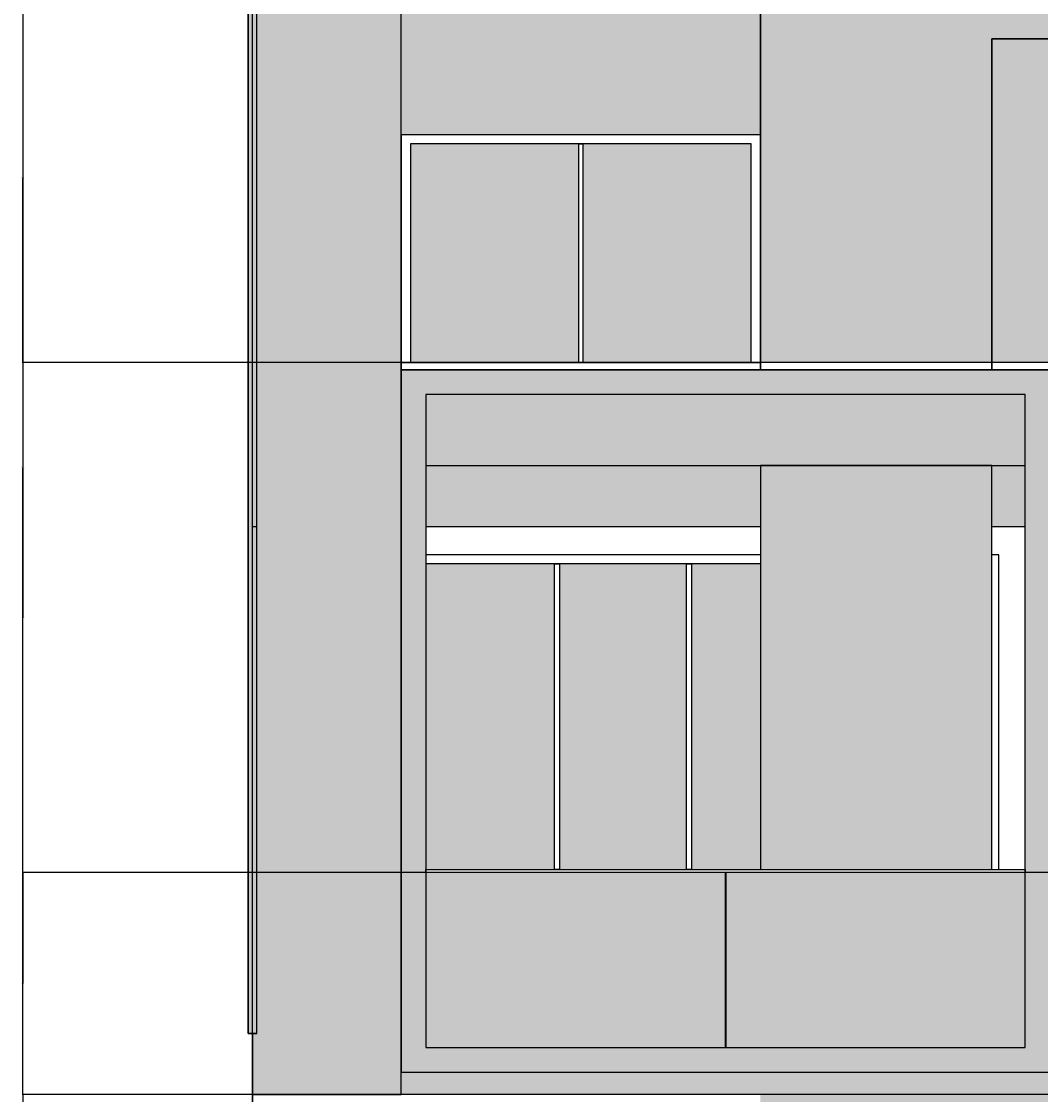
# Model space of a CAD drawing. Units: feet. Extents: x 2193 to 3502, y 890 to 1601.
# Tile 2 of 17: x 2193 to 2466, y 1073 to 1360. Entities that reach past the tile are written whole.
import ezdxf

# ---------------------------------------------------------------- set-up
doc = ezdxf.new("R2010")
doc.units = ezdxf.units.FT
for name, color, linetype, lineweight in [('A-ANNO-DIMS', 2, 'Continuous', 18), ('A-ELEV', 7, 'Continuous', 25), ('A-ELEV-PATT', 8, 'Continuous', 13)]:
    doc.layers.add(name, color=color, linetype=linetype, lineweight=lineweight)
doc.styles.get("Standard").update_dxf_attribs({"font": 'arial.ttf'})
doc.dimstyles.get("Standard").update_dxf_attribs({"dimtxt": 0.18, "dimasz": 0.18, "dimexe": 0.18, "dimexo": 0.0625, "dimgap": 0.09, "dimtad": 0, "dimtih": 1, "dimtoh": 1, "dimdec": 0, "dimzin": 0, "dimdsep": 46, "dimlunit": 3, "dimtxsty": 'Standard', "dimcen": 0.09, "dimadec": 0, "dimazin": 0, "dimtfac": 1, "dimtdec": 0, "dimtofl": 0, "dimtmove": 0, "dimatfit": 3, "dimfxl": 1, "dimtolj": 1, "dimtzin": 0, "dimarcsym": 0})

# ---------------------------------------------------------------- blocks, each defined once
blk = doc.blocks.new('*D19')
at = {"layer": 'A-ANNO-DIMS', "color": 0, "lineweight": -2, "transparency": 16777216}
for p, q in [((2934.31, 1073.03), (2193.56, 1073.03)), ((2193.74, 1072.85), (2193.74, 1012.11)), ((2193.74, 951), (2193.74, 1011.75)), ((2934.31, 950.82), (2193.56, 950.82))]:
    blk.add_line(p, q, dxfattribs=at)
at = {"layer": 'A-ANNO-DIMS', "color": 0, "transparency": 16777216}
for points in [[(2193.71, 1072.85), (2193.77, 1072.85), (2193.74, 1073.03)], [(2193.71, 951), (2193.77, 951), (2193.74, 950.82)]]:
    blk.add_solid(points, dxfattribs=at)
at = {"layer": 'Defpoints', "color": 0, "transparency": 16777216}
for p in [(2193.74, 1073.03), (2934.37, 1073.03), (2934.37, 950.82)]:
    blk.add_point(p, dxfattribs=at)
at = {"layer": 'A-ANNO-DIMS', "color": 0, "transparency": 16777216, "insert": (2193.74, 1011.93), "char_height": 0.18, "attachment_point": 5}
blk.add_mtext('\\A1;122.2', dxfattribs=at)
blk = doc.blocks.new('*D20')
at = {"layer": 'A-ANNO-DIMS', "color": 0, "lineweight": -2, "transparency": 16777216}
for p, q in [((2933.15, 1408.48), (2193.56, 1408.48)), ((2193.74, 1408.3), (2193.74, 1240.94)), ((2193.74, 1073.21), (2193.74, 1240.57)), ((2934.31, 1073.03), (2193.56, 1073.03))]:
    blk.add_line(p, q, dxfattribs=at)
at = {"layer": 'A-ANNO-DIMS', "color": 0, "transparency": 16777216}
for points in [[(2193.71, 1408.3), (2193.77, 1408.3), (2193.74, 1408.48)], [(2193.71, 1073.21), (2193.77, 1073.21), (2193.74, 1073.03)]]:
    blk.add_solid(points, dxfattribs=at)
at = {"layer": 'Defpoints', "color": 0, "transparency": 16777216}
for p in [(2193.74, 1408.48), (2933.21, 1408.48), (2934.37, 1073.03)]:
    blk.add_point(p, dxfattribs=at)
at = {"layer": 'A-ANNO-DIMS', "color": 0, "transparency": 16777216, "insert": (2193.74, 1240.76), "char_height": 0.18, "attachment_point": 5}
blk.add_mtext('\\A1;335.45', dxfattribs=at)
blk = doc.blocks.new('*D26')
at = {"layer": 'A-ANNO-DIMS', "color": 0, "lineweight": -2, "transparency": 16777216}
for p, q in [((2255.16, 950.89), (2255.16, 1601.47)), ((2255.34, 1601.29), (2507.42, 1601.29)), ((2760.29, 1601.29), (2508.21, 1601.29)), ((2760.47, 1541.11), (2760.47, 1601.47))]:
    blk.add_line(p, q, dxfattribs=at)
at = {"layer": 'A-ANNO-DIMS', "color": 0, "transparency": 16777216}
for points in [[(2255.34, 1601.32), (2255.34, 1601.26), (2255.16, 1601.29)], [(2760.29, 1601.32), (2760.29, 1601.26), (2760.47, 1601.29)]]:
    blk.add_solid(points, dxfattribs=at)
at = {"layer": 'Defpoints', "color": 0, "transparency": 16777216}
for p in [(2760.47, 1601.29), (2760.47, 1541.04), (2255.16, 950.82)]:
    blk.add_point(p, dxfattribs=at)
at = {"layer": 'A-ANNO-DIMS', "color": 0, "transparency": 16777216, "insert": (2507.82, 1601.29), "char_height": 0.18, "attachment_point": 5}
blk.add_mtext('\\A1;505.3', dxfattribs=at)
blk = doc.blocks.new('*D32')
at = {"layer": 'A-ANNO-DIMS', "color": 0, "lineweight": -2, "transparency": 16777216}
for p, q in [((2255.09, 1073.03), (2193.56, 1073.03)), ((2193.74, 1072.85), (2193.74, 1012.11)), ((2193.74, 951), (2193.74, 1011.75)), ((2255.09, 950.82), (2193.56, 950.82))]:
    blk.add_line(p, q, dxfattribs=at)
at = {"layer": 'A-ANNO-DIMS', "color": 0, "transparency": 16777216}
for points in [[(2193.71, 1072.85), (2193.77, 1072.85), (2193.74, 1073.03)], [(2193.71, 951), (2193.77, 951), (2193.74, 950.82)]]:
    blk.add_solid(points, dxfattribs=at)
at = {"layer": 'Defpoints', "color": 0, "transparency": 16777216}
for p in [(2193.74, 1073.03), (2255.16, 1073.03), (2255.16, 950.82)]:
    blk.add_point(p, dxfattribs=at)
at = {"layer": 'A-ANNO-DIMS', "color": 0, "transparency": 16777216, "insert": (2193.74, 1011.93), "char_height": 0.18, "attachment_point": 5}
blk.add_mtext('\\A1;122.2', dxfattribs=at)
blk = doc.blocks.new('*D33')
at = {"layer": 'A-ANNO-DIMS', "color": 0, "lineweight": -2, "transparency": 16777216}
for p, q in [((2253.93, 1408.48), (2193.56, 1408.48)), ((2193.74, 1408.3), (2193.74, 1240.94)), ((2193.74, 1073.21), (2193.74, 1240.57)), ((2255.09, 1073.03), (2193.56, 1073.03))]:
    blk.add_line(p, q, dxfattribs=at)
at = {"layer": 'A-ANNO-DIMS', "color": 0, "transparency": 16777216}
for points in [[(2193.71, 1408.3), (2193.77, 1408.3), (2193.74, 1408.48)], [(2193.71, 1073.21), (2193.77, 1073.21), (2193.74, 1073.03)]]:
    blk.add_solid(points, dxfattribs=at)
at = {"layer": 'Defpoints', "color": 0, "transparency": 16777216}
for p in [(2193.74, 1408.48), (2253.99, 1408.48), (2255.16, 1073.03)]:
    blk.add_point(p, dxfattribs=at)
at = {"layer": 'A-ANNO-DIMS', "color": 0, "transparency": 16777216, "insert": (2193.74, 1240.76), "char_height": 0.18, "attachment_point": 5}
blk.add_mtext('\\A1;335.45', dxfattribs=at)
blk = doc.blocks.new('*D35')
at = {"layer": 'A-ANNO-DIMS', "color": 0, "lineweight": -2, "transparency": 16777216}
for p, q in [((2980.65, 1132.39), (2193.56, 1132.39)), ((2193.74, 1132.21), (2193.74, 1102.89)), ((2193.74, 1073.21), (2193.74, 1102.53)), ((2934.31, 1073.03), (2193.56, 1073.03))]:
    blk.add_line(p, q, dxfattribs=at)
at = {"layer": 'A-ANNO-DIMS', "color": 0, "transparency": 16777216}
for points in [[(2193.71, 1132.21), (2193.77, 1132.21), (2193.74, 1132.39)], [(2193.71, 1073.21), (2193.77, 1073.21), (2193.74, 1073.03)]]:
    blk.add_solid(points, dxfattribs=at)
at = {"layer": 'Defpoints', "color": 0, "transparency": 16777216}
for p in [(2193.74, 1132.39), (2980.72, 1132.39), (2934.37, 1073.03)]:
    blk.add_point(p, dxfattribs=at)
at = {"layer": 'A-ANNO-DIMS', "color": 0, "transparency": 16777216, "insert": (2193.74, 1102.71), "char_height": 0.18, "attachment_point": 5}
blk.add_mtext('\\A1;59.36', dxfattribs=at)
blk = doc.blocks.new('*D36')
at = {"layer": 'A-ANNO-DIMS', "color": 0, "lineweight": -2, "transparency": 16777216}
for p, q in [((2974.05, 1268.66), (2193.56, 1268.66)), ((2193.74, 1268.48), (2193.74, 1200.71)), ((2193.74, 1132.57), (2193.74, 1200.34)), ((2980.65, 1132.39), (2193.56, 1132.39))]:
    blk.add_line(p, q, dxfattribs=at)
at = {"layer": 'A-ANNO-DIMS', "color": 0, "transparency": 16777216}
for points in [[(2193.71, 1268.48), (2193.77, 1268.48), (2193.74, 1268.66)], [(2193.71, 1132.57), (2193.77, 1132.57), (2193.74, 1132.39)]]:
    blk.add_solid(points, dxfattribs=at)
at = {"layer": 'Defpoints', "color": 0, "transparency": 16777216}
for p in [(2193.74, 1268.66), (2974.12, 1268.66), (2980.72, 1132.39)]:
    blk.add_point(p, dxfattribs=at)
at = {"layer": 'A-ANNO-DIMS', "color": 0, "transparency": 16777216, "insert": (2193.74, 1200.53), "char_height": 0.18, "attachment_point": 5}
blk.add_mtext('\\A1;136.27', dxfattribs=at)
blk = doc.blocks.new('*D37')
at = {"layer": 'A-ANNO-DIMS', "color": 0, "lineweight": -2, "transparency": 16777216}
for p, q in [((2974.05, 1367.57), (2193.56, 1367.57)), ((2193.74, 1367.39), (2193.74, 1318.3)), ((2193.74, 1268.84), (2193.74, 1317.93)), ((2974.05, 1268.66), (2193.56, 1268.66))]:
    blk.add_line(p, q, dxfattribs=at)
at = {"layer": 'A-ANNO-DIMS', "color": 0, "transparency": 16777216}
for points in [[(2193.71, 1367.39), (2193.77, 1367.39), (2193.74, 1367.57)], [(2193.71, 1268.84), (2193.77, 1268.84), (2193.74, 1268.66)]]:
    blk.add_solid(points, dxfattribs=at)
at = {"layer": 'Defpoints', "color": 0, "transparency": 16777216}
for p in [(2193.74, 1367.57), (2974.12, 1367.57), (2974.12, 1268.66)]:
    blk.add_point(p, dxfattribs=at)
at = {"layer": 'A-ANNO-DIMS', "color": 0, "transparency": 16777216, "insert": (2193.74, 1318.12), "char_height": 0.18, "attachment_point": 5}
blk.add_mtext('\\A1;98.91', dxfattribs=at)

msp = doc.modelspace()

# ---------------------------------------------------------------- hatches: boundary and pattern name
at = {"layer": 'A-ELEV-PATT'}
h = msp.add_hatch(color=256, dxfattribs=at)
h.dxf.hatch_style = 1
h.paths.add_polyline_path([(2760.4733, 1512.3957), (2586.1736, 1512.3957), (2586.1736, 1502.0763), (2602.8648, 1502.0763), (2699.5726, 1502.0763), (2699.6322, 1502.0763), (2760.4733, 1502.0763)])
h.paths.add_polyline_path([(2760.4733, 1382.0763), (2275.0482, 1382.0763), (2275.0482, 1367.5739), (2745.971, 1367.5739), (2745.971, 1166.2327), (2760.4733, 1166.2327)])
h.paths.add_polyline_path([(2468.2854, 1266.7092), (2294.8992, 1266.7092), (2294.8992, 1079.031), (2468.2854, 1079.031)])
h.paths.add_polyline_path([(2301.4984, 1260.11), (2461.6863, 1260.11), (2461.6863, 1085.6301), (2301.4984, 1085.6301)], flags=16)
h.paths.add_polyline_path([(2452.7821, 1241.1967), (2452.7821, 1217.2819), (2454.6216, 1217.2819), (2454.6216, 1133.1367), (2461.6863, 1133.1367), (2461.6863, 1132.3937), (2381.7172, 1132.3937), (2381.7172, 1085.6301), (2381.4675, 1085.6301), (2381.4675, 1132.3937), (2301.4984, 1132.3937), (2301.4984, 1133.1367), (2301.4984, 1217.2819), (2390.8933, 1217.2819), (2390.8933, 1241.1967)], flags=0)
h.paths.add_polyline_path([(2372.4936, 1214.8367), (2372.4936, 1133.1367), (2371.1246, 1133.1367), (2371.1246, 1214.8367), (2337.2323, 1214.8367), (2337.2323, 1133.1367), (2335.8632, 1133.1367), (2335.8632, 1214.8367), (2337.2323, 1214.8367)], flags=0)
h = msp.add_hatch(color=256, dxfattribs=at)
h.dxf.hatch_style = 1
h.paths.add_polyline_path([(2390.8933, 1367.5739), (2294.8992, 1367.5739), (2294.8992, 1329.5765), (2390.8933, 1329.5765)])
h.paths.add_polyline_path([(2489.6169, 1055.3069), (2585.8844, 1055.3069), (2585.8844, 1032.1935), (2620.0491, 1032.1935), (2620.0491, 1073.031), (2452.7821, 1073.031), (2452.7821, 1032.1935), (2489.6169, 1032.1935)])
h.paths.add_polyline_path([(2754.7661, 1073.031), (2654.2841, 1073.031), (2654.2841, 1047.0961), (2754.7661, 1047.0961)])
h.paths.add_polyline_path([(2643.9681, 1484.1152), (2699.5726, 1484.1152), (2699.5726, 1502.0763), (2602.8648, 1502.0763), (2602.8648, 1408.4814), (2643.9681, 1408.4814)])
h.paths.add_polyline_path([(2699.6322, 1367.5739), (2646.2844, 1367.5739), (2646.2844, 1268.6599), (2647.1841, 1268.6599), (2647.1841, 1329.5765), (2699.6322, 1329.5765)])
h.paths.add_polyline_path([(2699.6322, 1224.865), (2616.5596, 1224.865), (2616.5596, 1133.8558), (2647.1841, 1133.8558), (2647.1841, 1194.7724), (2699.6322, 1194.7724)])
h = msp.add_hatch(color=256, dxfattribs=at)
h.dxf.hatch_style = 1
h.paths.add_polyline_path([(2256.3232, 1406.15), (2536.5416, 1406.15), (2536.5416, 1408.4814), (2253.9917, 1408.4814), (2253.9917, 1089.3627), (2255.1574, 1089.3627), (2256.3232, 1089.3627)])
h = msp.add_hatch(color=256, dxfattribs=at)
h.dxf.hatch_style = 1
h.paths.add_polyline_path([(2294.8992, 1367.5739), (2275.0482, 1367.5739), (2275.0482, 1382.0763), (2536.5416, 1382.0763), (2536.5416, 1406.15), (2256.3232, 1406.15), (2256.3232, 1089.3627), (2255.1574, 1089.3627), (2255.1574, 1073.031), (2294.8992, 1073.031)])
h.paths.add_polyline_path([(2517.7591, 1241.1967), (2468.2854, 1241.1967), (2468.2854, 1224.865), (2598.591, 1224.865), (2598.591, 1233.561), (2517.7591, 1233.561)])
h.paths.add_polyline_path([(2699.6322, 1241.1967), (2636.5184, 1241.1967), (2636.5184, 1233.561), (2616.5596, 1233.561), (2616.5596, 1224.865), (2699.6322, 1224.865)])
h.paths.add_polyline_path([(2615.4622, 1233.561), (2613.8564, 1233.561), (2613.8564, 1224.865), (2615.4622, 1224.865)])
h.paths.add_polyline_path([(2612.759, 1233.561), (2609.5836, 1233.561), (2609.5836, 1224.865), (2612.759, 1224.865)])
h.paths.add_polyline_path([(2608.4862, 1233.561), (2606.5316, 1233.561), (2606.5316, 1224.865), (2608.4862, 1224.865)])
h.paths.add_polyline_path([(2605.4342, 1233.561), (2602.5204, 1233.561), (2602.5204, 1224.865), (2605.4342, 1224.865)])
h.paths.add_polyline_path([(2601.423, 1233.561), (2599.6883, 1233.561), (2599.6883, 1224.865), (2601.423, 1224.865)])
h.paths.add_polyline_path([(2517.7591, 1089.3627), (2468.2854, 1089.3627), (2468.2854, 1079.031), (2294.8992, 1079.031), (2294.8992, 1073.031), (2390.8933, 1073.031), (2452.7821, 1073.031), (2760.4733, 1073.031), (2760.4733, 1089.3627), (2699.6322, 1089.3627), (2636.5184, 1089.3627), (2636.5184, 1081.7269), (2517.7591, 1081.7269)])
h = msp.add_hatch(color=256, dxfattribs=at)
h.dxf.hatch_style = 1
h.paths.add_polyline_path([(2576.3428, 1407.7384), (2536.5416, 1407.7384), (2536.5416, 1406.15), (2536.5416, 1382.0763), (2576.3428, 1382.0763)])
h.paths.add_polyline_path([(2627.3548, 1407.7384), (2576.5924, 1407.7384), (2576.5924, 1382.0763), (2627.3548, 1382.0763)])
h.paths.add_polyline_path([(2667.9236, 1407.7384), (2627.6045, 1407.7384), (2627.6045, 1382.0763), (2667.9236, 1382.0763)])
h.paths.add_polyline_path([(2699.6322, 1407.7384), (2668.1733, 1407.7384), (2668.1733, 1382.0763), (2699.6322, 1382.0763)])
h.paths.add_polyline_path([(2497.5717, 1323.2248), (2470.7305, 1323.2248), (2470.7305, 1271.105), (2497.5717, 1271.105)])
h.paths.add_polyline_path([(2577.3219, 1323.2248), (2500.599, 1323.2248), (2500.599, 1271.105), (2577.3219, 1271.105)])
h.paths.add_polyline_path([(2388.4482, 1327.1314), (2343.4244, 1327.1314), (2343.4244, 1268.6599), (2388.4482, 1268.6599)])
h.paths.add_polyline_path([(2342.3682, 1327.1314), (2297.3443, 1327.1314), (2297.3443, 1268.6599), (2342.3682, 1268.6599)])
h.paths.add_polyline_path([(2335.8632, 1214.8367), (2301.4984, 1214.8367), (2301.4984, 1133.1367), (2335.8632, 1133.1367)])
h.paths.add_polyline_path([(2371.1246, 1214.8367), (2337.2323, 1214.8367), (2337.2323, 1133.1367), (2371.1246, 1133.1367)])
h.paths.add_polyline_path([(2390.8933, 1214.8367), (2372.4936, 1214.8367), (2372.4936, 1133.1367), (2390.8933, 1133.1367)])
h.paths.add_polyline_path([(2577.3219, 1188.4208), (2500.599, 1188.4208), (2500.599, 1136.3009), (2577.3219, 1136.3009)])
h.paths.add_polyline_path([(2497.5717, 1188.4208), (2470.7305, 1188.4208), (2470.7305, 1136.3009), (2497.5717, 1136.3009)])
h.paths.add_polyline_path([(2381.4675, 1132.3937), (2301.4984, 1132.3937), (2301.4984, 1085.6301), (2381.4675, 1085.6301)])
h.paths.add_polyline_path([(2461.6863, 1132.3937), (2381.7172, 1132.3937), (2381.7172, 1085.6301), (2461.6863, 1085.6301)])
h.paths.add_polyline_path([(2494.0463, 1133.1128), (2468.2854, 1133.1128), (2468.2854, 1089.3627), (2494.0463, 1089.3627)])
h.paths.add_polyline_path([(2517.7591, 1133.1128), (2494.296, 1133.1128), (2494.296, 1089.3627), (2517.7591, 1089.3627)])
h.paths.add_polyline_path([(2667.9236, 1133.1128), (2636.5184, 1133.1128), (2636.5184, 1089.3627), (2667.9236, 1089.3627)])
h.paths.add_polyline_path([(2699.6322, 1133.1128), (2668.1733, 1133.1128), (2668.1733, 1089.3627), (2699.6322, 1089.3627)])
h.paths.add_polyline_path([(2651.839, 1070.5859), (2638.7977, 1070.5859), (2638.7977, 1047.0961), (2651.839, 1047.0961)])
h.paths.add_polyline_path([(2637.6317, 1070.5859), (2625.7563, 1070.5859), (2625.7563, 1047.0961), (2637.6317, 1047.0961)])
h.paths.add_polyline_path([(2583.4393, 1052.8618), (2515.9216, 1052.8618), (2515.9216, 1032.1935), (2583.4393, 1032.1935)])
h.paths.add_polyline_path([(2514.4293, 1052.8618), (2492.062, 1052.8618), (2492.062, 1032.1935), (2514.4293, 1032.1935)])
h.paths.add_polyline_path([(2388.4482, 1038.8658), (2348.7682, 1038.8658), (2348.7682, 988.9597), (2388.4482, 988.9597)])
h.paths.add_polyline_path([(2346.3231, 1038.8658), (2309.0883, 1038.8658), (2309.0883, 988.9597), (2346.3231, 988.9597)])
h.paths.add_polyline_path([(2667.9236, 1267.9169), (2636.5184, 1267.9169), (2636.5184, 1241.1967), (2667.9236, 1241.1967)])
h.paths.add_polyline_path([(2699.6322, 1267.9169), (2668.1733, 1267.9169), (2668.1733, 1241.1967), (2699.6322, 1241.1967)])
h.paths.add_polyline_path([(2517.7591, 1267.9169), (2494.296, 1267.9169), (2494.296, 1241.1967), (2517.7591, 1241.1967)])
h.paths.add_polyline_path([(2494.0463, 1267.9169), (2468.2854, 1267.9169), (2468.2854, 1266.7092), (2468.2854, 1241.1967), (2494.0463, 1241.1967)])
h = msp.add_hatch(color=256, dxfattribs=at)
h.dxf.hatch_style = 1
h.paths.add_polyline_path([(2452.7821, 1355.2199), (2622.9814, 1355.2199), (2622.9814, 1268.6599), (2646.2844, 1268.6599), (2646.2844, 1367.5739), (2390.8933, 1367.5739), (2390.8933, 1268.6599), (2452.7821, 1268.6599)])
h.paths.add_polyline_path([(2452.7821, 1016.4), (2431.9134, 1016.4), (2431.9134, 1032.1935), (2452.7821, 1032.1935), (2452.7821, 1073.031), (2390.8933, 1073.031), (2390.8933, 956.8829), (2452.7821, 956.8829)])
h.paths.add_polyline_path([(2452.7821, 1241.1967), (2390.8933, 1241.1967), (2390.8933, 1133.1367), (2452.7821, 1133.1367)])
h.paths.add_polyline_path([(2636.5184, 1267.9169), (2517.7591, 1267.9169), (2517.7591, 1233.561), (2598.591, 1233.561), (2598.591, 1249.8256), (2599.6883, 1249.8256), (2599.6883, 1233.561), (2601.423, 1233.561), (2601.423, 1247.0422), (2602.5204, 1247.0422), (2602.5204, 1233.561), (2605.4342, 1233.561), (2605.4342, 1250.4403), (2606.5316, 1250.4403), (2606.5316, 1233.561), (2608.4862, 1233.561), (2608.4862, 1248.4363), (2609.5836, 1248.4363), (2609.5836, 1233.561), (2612.759, 1233.561), (2612.759, 1243.2956), (2613.8564, 1243.2956), (2613.8564, 1233.561), (2615.4622, 1233.561), (2615.4622, 1249.6561), (2616.5596, 1249.6561), (2616.5596, 1233.561), (2636.5184, 1233.561)])
h.paths.add_polyline_path([(2601.423, 1133.1128), (2599.6883, 1133.1128), (2599.6883, 1115.2331), (2598.591, 1115.2331), (2598.591, 1133.1128), (2517.7591, 1133.1128), (2517.7591, 1081.7269), (2636.5184, 1081.7269), (2636.5184, 1133.1128), (2616.5596, 1133.1128), (2616.5596, 1115.0637), (2615.4622, 1115.0637), (2615.4622, 1133.1128), (2613.8564, 1133.1128), (2613.8564, 1108.7032), (2612.759, 1108.7032), (2612.759, 1133.1128), (2609.5836, 1133.1128), (2609.5836, 1113.8439), (2608.4862, 1113.8439), (2608.4862, 1133.1128), (2606.5316, 1133.1128), (2606.5316, 1115.8479), (2605.4342, 1115.8479), (2605.4342, 1133.1128), (2602.5204, 1133.1128), (2602.5204, 1112.4498), (2601.423, 1112.4498)])
h = msp.add_hatch(color=256, dxfattribs=at)
h.dxf.hatch_style = 1
h.paths.add_polyline_path([(2622.9814, 1355.2199), (2452.7821, 1355.2199), (2452.7821, 1268.6599), (2468.2854, 1268.6599), (2468.2854, 1325.6699), (2579.767, 1325.6699), (2579.767, 1268.6599), (2622.9814, 1268.6599)])
h.paths.add_polyline_path([(2598.591, 1224.865), (2468.2854, 1224.865), (2468.2854, 1190.8659), (2579.767, 1190.8659), (2579.767, 1133.8558), (2598.591, 1133.8558)])
h.paths.add_polyline_path([(2390.8933, 1241.1967), (2301.4984, 1241.1967), (2301.4984, 1224.865), (2390.8933, 1224.865)])
h.paths.add_polyline_path([(3070.1101, 1073.031), (2940.0814, 1073.031), (2940.0814, 956.5285), (2940.6598, 956.8829), (3070.1101, 956.8829), (3070.1101, 986.5146), (2985.8599, 986.5146), (2985.8599, 1041.3109), (3070.1101, 1041.3109)])
h = msp.add_hatch(color=256, dxfattribs=at)
h.dxf.hatch_style = 1
h.paths.add_polyline_path([(2461.6863, 1260.11), (2301.4984, 1260.11), (2301.4984, 1241.1967), (2461.6863, 1241.1967)])
h = msp.add_hatch(color=256, dxfattribs=at)
h.dxf.hatch_style = 1
h.paths.add_polyline_path([(2461.6863, 1241.1967), (2452.7821, 1241.1967), (2452.7821, 1224.865), (2461.6863, 1224.865)])

# ---------------------------------------------------------------- linework, layer by layer
at = {"layer": 'A-ELEV'}
for p, q in [((2452.7821, 1355.2199), (2622.9814, 1355.2199)), ((2301.4984, 1241.1967), (2461.6863, 1241.1967)), ((2301.4984, 1241.1967), (2461.6863, 1241.1967)), ((2255.1574, 1224.865), (2256.3232, 1224.865)), ((2301.4984, 1224.865), (2390.8933, 1224.865)), ((2301.4984, 1224.865), (2390.8933, 1224.865)), ((2452.7821, 1224.865), (2461.6863, 1224.865)), ((2452.7821, 1224.865), (2461.6863, 1224.865)), ((2255.1574, 953.031), (2255.1574, 1089.3627)), ((2255.1574, 1089.3627), (2256.3232, 1089.3627))]:
    msp.add_line(p, q, dxfattribs=at)
for points in [[(2256.3232, 1406.15), (2536.5416, 1406.15), (2536.5416, 1408.4814), (2253.9917, 1408.4814), (2253.9917, 1089.3627), (2255.1574, 1089.3627), (2256.3232, 1089.3627)], [(2294.8992, 1268.6599), (2390.8933, 1268.6599), (2390.8933, 1329.5765), (2294.8992, 1329.5765)], [(2294.8992, 1268.6599), (2390.8933, 1268.6599), (2390.8933, 1329.5765), (2294.8992, 1329.5765)], [(2342.3682, 1327.1314), (2343.4244, 1327.1314), (2343.4244, 1268.6599), (2342.3682, 1268.6599)], [(2342.3682, 1327.1314), (2343.4244, 1327.1314), (2343.4244, 1268.6599), (2342.3682, 1268.6599)], [(2294.8992, 1266.7092), (2468.2854, 1266.7092), (2468.2854, 1268.6599), (2294.8992, 1268.6599)], [(2294.8992, 1266.7092), (2468.2854, 1266.7092), (2468.2854, 1268.6599), (2294.8992, 1268.6599)], [(2294.8992, 1079.031), (2468.2854, 1079.031), (2468.2854, 1266.7092), (2294.8992, 1266.7092)], [(2294.8992, 1079.031), (2468.2854, 1079.031), (2468.2854, 1266.7092), (2294.8992, 1266.7092)], [(2301.4984, 1085.6301), (2461.6863, 1085.6301), (2461.6863, 1260.11), (2301.4984, 1260.11)], [(2301.4984, 1085.6301), (2461.6863, 1085.6301), (2461.6863, 1260.11), (2301.4984, 1260.11)], [(2335.8632, 1214.8367), (2337.2323, 1214.8367), (2337.2323, 1133.1367), (2335.8632, 1133.1367)], [(2335.8632, 1214.8367), (2337.2323, 1214.8367), (2337.2323, 1133.1367), (2335.8632, 1133.1367)], [(2371.1246, 1214.8367), (2372.4936, 1214.8367), (2372.4936, 1133.1367), (2371.1246, 1133.1367)], [(2371.1246, 1214.8367), (2372.4936, 1214.8367), (2372.4936, 1133.1367), (2371.1246, 1133.1367)], [(2301.4984, 1133.1367), (2461.6863, 1133.1367), (2461.6863, 1132.3937), (2301.4984, 1132.3937)], [(2301.4984, 1133.1367), (2461.6863, 1133.1367), (2461.6863, 1132.3937), (2301.4984, 1132.3937)], [(2381.4675, 1085.6301), (2381.7172, 1085.6301), (2381.7172, 1132.3937), (2381.4675, 1132.3937)], [(2381.4675, 1085.6301), (2381.7172, 1085.6301), (2381.7172, 1132.3937), (2381.4675, 1132.3937)]]:
    msp.add_lwpolyline(points, close=True, dxfattribs=at)
for points in [[(2255.1574, 1089.3627), (2253.9917, 1089.3627), (2253.9917, 1408.4814), (2255.1574, 1408.4814)], [(2255.1574, 1089.3627), (2256.3232, 1089.3627), (2256.3232, 1406.15)], [(2256.3232, 1089.3627), (2255.1574, 1089.3627), (2255.1574, 1073.031), (2294.8992, 1073.031), (2294.8992, 1367.5739), (2536.5416, 1367.5739), (2646.2844, 1367.5739)], [(2255.1574, 1089.3627), (2255.1574, 1073.031), (2294.8992, 1073.031), (2294.8992, 1367.5739)], [(2622.9814, 1367.5739), (2646.2844, 1367.5739), (2646.2844, 1268.6599), (2622.9814, 1268.6599), (2622.9814, 1355.2199), (2452.7821, 1355.2199), (2452.7821, 1266.7092), (2390.8933, 1266.7092), (2390.8933, 1367.5739)], [(2390.8933, 1367.5739), (2390.8933, 1266.7092), (2452.7821, 1266.7092), (2452.7821, 1355.2199)], [(2388.4482, 1268.6599), (2388.4482, 1327.1314), (2297.3443, 1327.1314), (2297.3443, 1268.6599)], [(2388.4482, 1268.6599), (2388.4482, 1327.1314), (2297.3443, 1327.1314), (2297.3443, 1268.6599)], [(2452.7821, 1133.1367), (2452.7821, 1241.1967), (2390.8933, 1241.1967), (2390.8933, 1133.1367)], [(2452.7821, 1133.1367), (2452.7821, 1241.1967), (2390.8933, 1241.1967), (2390.8933, 1133.1367)], [(2390.8933, 1217.2819), (2301.4984, 1217.2819), (2301.4984, 1133.1367)], [(2390.8933, 1217.2819), (2301.4984, 1217.2819), (2301.4984, 1133.1367)], [(2454.6216, 1133.1367), (2454.6216, 1217.2819), (2452.7821, 1217.2819)], [(2454.6216, 1133.1367), (2454.6216, 1217.2819), (2452.7821, 1217.2819)], [(2390.8933, 1214.8367), (2301.4984, 1214.8367)], [(2390.8933, 1214.8367), (2301.4984, 1214.8367)], [(2255.1574, 1089.3627), (2255.1574, 953.031), (2261.443, 956.8829), (2461.0056, 956.8829)]]:
    msp.add_lwpolyline(points, dxfattribs=at)

# ---------------------------------------------------------------- dimensions: what is measured, and where the dimension line sits
at = {"layer": 'A-ANNO-DIMS'}
dim = msp.add_linear_dim(base=(2760.4733, 1601.2941), p1=(2255.1574, 950.8228), p2=(2760.4733, 1541.0441), dimstyle='Standard', override={"dimdec": 1, "dimlfac": 1, "dimrnd": 0, "dimzin": 0, "dimdsep": 46, "dimlunit": 2}, dxfattribs=at)
dim.commit()
dim.dimension.update_dxf_attribs({"geometry": '*D26', "text_midpoint": (2507.8154, 1601.2941)})
for base, p1, p2, override, picture, middle in [((2193.7417, 1408.4814), (2934.3742, 1073.031), (2933.2085, 1408.4814), {"dimdec": 2, "dimlfac": 1, "dimrnd": 0, "dimzin": 0, "dimdsep": 46, "dimlunit": 2}, '*D20', (2193.7417, 1240.7562)), ((2193.7417, 1408.4814), (2255.1574, 1073.031), (2253.9917, 1408.4814), {"dimdec": 2, "dimlfac": 1, "dimrnd": 0, "dimzin": 0, "dimdsep": 46, "dimlunit": 2}, '*D33', (2193.7417, 1240.7562)), ((2193.7417, 1367.5739), (2974.116, 1268.6599), (2974.116, 1367.5739), {"dimdec": 2, "dimlfac": 1, "dimrnd": 0, "dimzin": 0, "dimdsep": 46, "dimlunit": 2}, '*D37', (2193.7417, 1318.1169)), ((2193.7417, 1268.6599), (2980.7151, 1132.3937), (2974.116, 1268.6599), {"dimdec": 2, "dimlfac": 1, "dimrnd": 0, "dimzin": 0, "dimdsep": 46, "dimlunit": 2}, '*D36', (2193.7417, 1200.5268)), ((2193.7417, 1132.3937), (2934.3742, 1073.031), (2980.7151, 1132.3937), {"dimdec": 2, "dimlfac": 1, "dimrnd": 0, "dimzin": 0, "dimdsep": 46, "dimlunit": 2}, '*D35', (2193.7417, 1102.7124)), ((2193.7417, 1073.031), (2934.3742, 950.8228), (2934.3742, 1073.031), {"dimdec": 1, "dimlfac": 1, "dimrnd": 0, "dimzin": 0, "dimdsep": 46, "dimlunit": 2}, '*D19', (2193.7417, 1011.9269)), ((2193.7417, 1073.031), (2255.1574, 950.8228), (2255.1574, 1073.031), {"dimdec": 1, "dimlfac": 1, "dimrnd": 0, "dimzin": 0, "dimdsep": 46, "dimlunit": 2}, '*D32', (2193.7417, 1011.9269))]:
    dim = msp.add_linear_dim(base=base, p1=p1, p2=p2, angle=90, dimstyle='Standard', override=override, dxfattribs=at)
    dim.commit()
    dim.dimension.update_dxf_attribs({"geometry": picture, "text_midpoint": middle})

doc.saveas('drawing.dxf')
